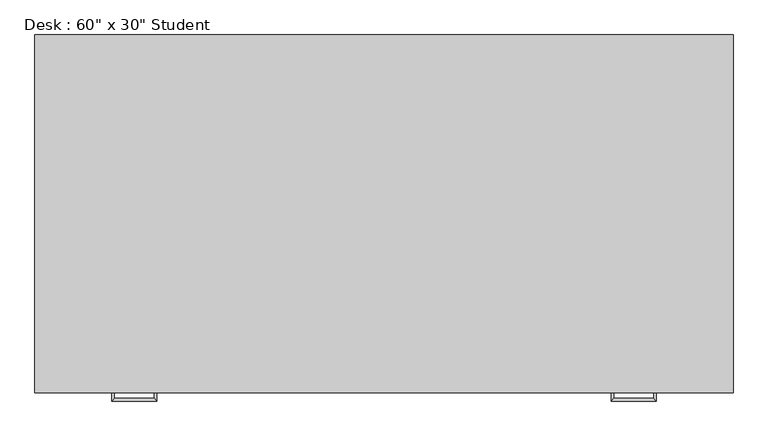
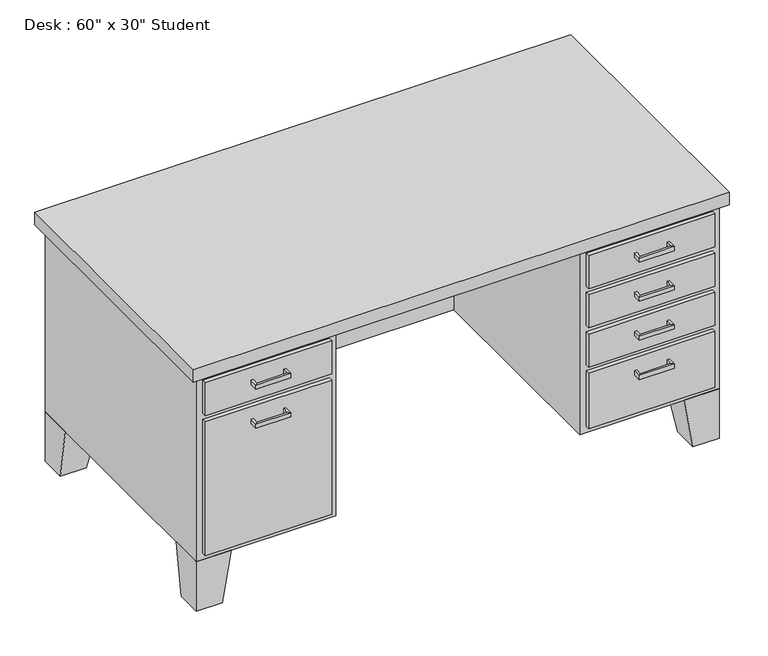
"""IFC4 building model written with IfcOpenShell, lengths in millimetres: furniture geometry."""

from ifc_helpers import new_model, si_unit, frame, origin, place, context, project, spatial, polyline, outline, extrude, faceted_brep, source, transform, mapped, element, save


def furniture_013ab306(model_context):
    return source(origin(), model_context, "Body", "SolidModel", [
        extrude(outline(polyline([(19.05, 0.0), (387.35, 0.0), (387.35, -12.7), (19.05, -12.7), (19.05, 0.0)])), frame((0.0, 0.0, 603.25), z_axis=(0.0, 0.0, 1.0), x_axis=(1.0, 0.0, 0.0)), (0.0, 0.0, 1.0), 101.6),
        extrude(outline(polyline([(19.05, 0.0), (387.35, 0.0), (387.35, -12.7), (19.05, -12.7), (19.05, 0.0)])), frame((0.0, 0.0, 171.45), z_axis=(0.0, 0.0, 1.0), x_axis=(1.0, 0.0, 0.0)), (0.0, 0.0, 1.0), 412.75),
        extrude(outline(polyline([(1136.65, 0.0), (1504.95, 0.0), (1504.95, -12.7), (1136.65, -12.7), (1136.65, 0.0)])), frame((0.0, 0.0, 603.25), z_axis=(0.0, 0.0, 1.0), x_axis=(1.0, 0.0, 0.0)), (0.0, 0.0, 1.0), 101.6),
        extrude(outline(polyline([(1136.65, 0.0), (1504.95, 0.0), (1504.95, -12.7), (1136.65, -12.7), (1136.65, 0.0)])), frame((0.0, 0.0, 171.45), z_axis=(0.0, 0.0, 1.0), x_axis=(1.0, 0.0, 0.0)), (0.0, 0.0, 1.0), 171.45),
        extrude(outline(polyline([(1136.65, 0.0), (1504.95, 0.0), (1504.95, -12.7), (1136.65, -12.7), (1136.65, 0.0)])), frame((0.0, 0.0, 482.6), z_axis=(0.0, 0.0, 1.0), x_axis=(1.0, 0.0, 0.0)), (0.0, 0.0, 1.0), 101.6),
        extrude(outline(polyline([(1136.65, 0.0), (1504.95, 0.0), (1504.95, -12.7), (1136.65, -12.7), (1136.65, 0.0)])), frame((0.0, 0.0, 361.95), z_axis=(0.0, 0.0, 1.0), x_axis=(1.0, 0.0, 0.0)), (0.0, 0.0, 1.0), 101.6),
        faceted_brep([(101.6, 0.0, 152.4), (101.6, 101.6, 152.4), (0.0, 101.6, 152.4), (0.0, 0.0, 152.4), (76.2, 0.0, 0.0), (0.0, 0.0, 0.0), (0.0, 76.2, 0.0), (76.2, 76.2, 0.0)], [[[0, 1, 2, 3]], [[4, 5, 6, 7]], [[4, 7, 1, 0]], [[7, 6, 2, 1]], [[6, 5, 3, 2]], [[5, 4, 0, 3]]]),
        faceted_brep([(101.6, 762.0, 152.4), (0.0, 762.0, 152.4), (0.0, 660.4, 152.4), (101.6, 660.4, 152.4), (76.2, 762.0, 0.0), (76.2, 685.8, 0.0), (0.0, 685.8, 0.0), (0.0, 762.0, 0.0)], [[[0, 1, 2, 3]], [[4, 5, 6, 7]], [[4, 7, 1, 0]], [[7, 6, 2, 1]], [[6, 5, 3, 2]], [[5, 4, 0, 3]]]),
        faceted_brep([(1422.4, 762.0, 152.4), (1422.4, 660.4, 152.4), (1524.0, 660.4, 152.4), (1524.0, 762.0, 152.4), (1447.8, 762.0, 0.0), (1524.0, 762.0, 0.0), (1524.0, 685.8, 0.0), (1447.8, 685.8, 0.0)], [[[0, 1, 2, 3]], [[4, 5, 6, 7]], [[4, 7, 1, 0]], [[7, 6, 2, 1]], [[6, 5, 3, 2]], [[5, 4, 0, 3]]]),
        faceted_brep([(1422.4, 0.0, 152.4), (1524.0, 0.0, 152.4), (1524.0, 101.6, 152.4), (1422.4, 101.6, 152.4), (1447.8, 0.0, 0.0), (1447.8, 76.2, 0.0), (1524.0, 76.2, 0.0), (1524.0, 0.0, 0.0)], [[[0, 1, 2, 3]], [[4, 5, 6, 7]], [[4, 7, 1, 0]], [[7, 6, 2, 1]], [[6, 5, 3, 2]], [[5, 4, 0, 3]]]),
        extrude(outline(polyline([(-19.05, -19.05), (-19.05, 781.05), (1543.05, 781.05), (1543.05, -19.05), (-19.05, -19.05)])), frame((0.0, 0.0, 723.9), z_axis=(0.0, 0.0, 1.0), x_axis=(1.0, 0.0, 0.0)), (0.0, 0.0, 1.0), 38.1),
        extrude(outline(polyline([(1117.6, 0.0), (1117.6, 635.0), (406.4, 635.0), (406.4, 0.0), (0.0, 0.0), (0.0, 762.0), (1524.0, 762.0), (1524.0, 0.0), (1117.6, 0.0)])), frame((0.0, 0.0, 152.4), z_axis=(0.0, 0.0, 1.0), x_axis=(1.0, 0.0, 0.0)), (0.0, 0.0, 1.0), 571.5),
        faceted_brep([(158.75, -12.7, 546.1), (158.75, -12.7, 533.4), (152.4, -12.7, 533.4), (152.4, -12.7, 546.1), (158.75, -31.75, 546.1), (158.75, -31.75, 533.4), (152.4, -38.1, 533.4), (152.4, -38.1, 546.1), (247.65, -31.75, 546.1), (247.65, -31.75, 533.4), (254.0, -38.1, 533.4), (254.0, -38.1, 546.1), (247.65, -12.7, 546.1), (254.0, -12.7, 546.1), (254.0, -12.7, 533.4), (247.65, -12.7, 533.4)], [[[0, 1, 2, 3]], [[1, 0, 4, 5]], [[2, 1, 5, 6]], [[3, 2, 6, 7]], [[0, 3, 7, 4]], [[5, 4, 8, 9]], [[6, 5, 9, 10]], [[7, 6, 10, 11]], [[4, 7, 11, 8]], [[12, 13, 14, 15]], [[9, 8, 12, 15]], [[10, 9, 15, 14]], [[11, 10, 14, 13]], [[8, 11, 13, 12]]]),
        faceted_brep([(158.75, -12.7, 666.75), (158.75, -12.7, 654.05), (152.4, -12.7, 654.05), (152.4, -12.7, 666.75), (158.75, -31.75, 666.75), (158.75, -31.75, 654.05), (152.4, -38.1, 654.05), (152.4, -38.1, 666.75), (247.65, -31.75, 666.75), (247.65, -31.75, 654.05), (254.0, -38.1, 654.05), (254.0, -38.1, 666.75), (247.65, -12.7, 666.75), (254.0, -12.7, 666.75), (254.0, -12.7, 654.05), (247.65, -12.7, 654.05)], [[[0, 1, 2, 3]], [[1, 0, 4, 5]], [[2, 1, 5, 6]], [[3, 2, 6, 7]], [[0, 3, 7, 4]], [[5, 4, 8, 9]], [[6, 5, 9, 10]], [[7, 6, 10, 11]], [[4, 7, 11, 8]], [[12, 13, 14, 15]], [[9, 8, 12, 15]], [[10, 9, 15, 14]], [[11, 10, 14, 13]], [[8, 11, 13, 12]]]),
        faceted_brep([(1365.25, -12.7, 304.8), (1371.6, -12.7, 304.8), (1371.6, -12.7, 292.1), (1365.25, -12.7, 292.1), (1365.25, -31.75, 304.8), (1371.6, -38.1, 304.8), (1371.6, -38.1, 292.1), (1365.25, -31.75, 292.1), (1276.35, -31.75, 304.8), (1270.0, -38.1, 304.8), (1270.0, -38.1, 292.1), (1276.35, -31.75, 292.1), (1276.35, -12.7, 304.8), (1276.35, -12.7, 292.1), (1270.0, -12.7, 292.1), (1270.0, -12.7, 304.8)], [[[0, 1, 2, 3]], [[1, 0, 4, 5]], [[2, 1, 5, 6]], [[3, 2, 6, 7]], [[0, 3, 7, 4]], [[5, 4, 8, 9]], [[6, 5, 9, 10]], [[7, 6, 10, 11]], [[4, 7, 11, 8]], [[12, 13, 14, 15]], [[9, 8, 12, 15]], [[10, 9, 15, 14]], [[11, 10, 14, 13]], [[8, 11, 13, 12]]]),
        faceted_brep([(1365.25, -12.7, 425.45), (1371.6, -12.7, 425.45), (1371.6, -12.7, 412.75), (1365.25, -12.7, 412.75), (1365.25, -31.75, 425.45), (1371.6, -38.1, 425.45), (1371.6, -38.1, 412.75), (1365.25, -31.75, 412.75), (1276.35, -31.75, 425.45), (1270.0, -38.1, 425.45), (1270.0, -38.1, 412.75), (1276.35, -31.75, 412.75), (1276.35, -12.7, 425.45), (1276.35, -12.7, 412.75), (1270.0, -12.7, 412.75), (1270.0, -12.7, 425.45)], [[[0, 1, 2, 3]], [[1, 0, 4, 5]], [[2, 1, 5, 6]], [[3, 2, 6, 7]], [[0, 3, 7, 4]], [[5, 4, 8, 9]], [[6, 5, 9, 10]], [[7, 6, 10, 11]], [[4, 7, 11, 8]], [[12, 13, 14, 15]], [[9, 8, 12, 15]], [[10, 9, 15, 14]], [[11, 10, 14, 13]], [[8, 11, 13, 12]]]),
        faceted_brep([(1365.25, -12.7, 546.1), (1371.6, -12.7, 546.1), (1371.6, -12.7, 533.4), (1365.25, -12.7, 533.4), (1365.25, -31.75, 546.1), (1371.6, -38.1, 546.1), (1371.6, -38.1, 533.4), (1365.25, -31.75, 533.4), (1276.35, -31.75, 546.1), (1270.0, -38.1, 546.1), (1270.0, -38.1, 533.4), (1276.35, -31.75, 533.4), (1276.35, -12.7, 546.1), (1276.35, -12.7, 533.4), (1270.0, -12.7, 533.4), (1270.0, -12.7, 546.1)], [[[0, 1, 2, 3]], [[1, 0, 4, 5]], [[2, 1, 5, 6]], [[3, 2, 6, 7]], [[0, 3, 7, 4]], [[5, 4, 8, 9]], [[6, 5, 9, 10]], [[7, 6, 10, 11]], [[4, 7, 11, 8]], [[12, 13, 14, 15]], [[9, 8, 12, 15]], [[10, 9, 15, 14]], [[11, 10, 14, 13]], [[8, 11, 13, 12]]]),
        faceted_brep([(1365.25, -12.7, 666.75), (1371.6, -12.7, 666.75), (1371.6, -12.7, 654.05), (1365.25, -12.7, 654.05), (1365.25, -31.75, 666.75), (1371.6, -38.1, 666.75), (1371.6, -38.1, 654.05), (1365.25, -31.75, 654.05), (1276.35, -31.75, 666.75), (1270.0, -38.1, 666.75), (1270.0, -38.1, 654.05), (1276.35, -31.75, 654.05), (1276.35, -12.7, 666.75), (1276.35, -12.7, 654.05), (1270.0, -12.7, 654.05), (1270.0, -12.7, 666.75)], [[[0, 1, 2, 3]], [[1, 0, 4, 5]], [[2, 1, 5, 6]], [[3, 2, 6, 7]], [[0, 3, 7, 4]], [[5, 4, 8, 9]], [[6, 5, 9, 10]], [[7, 6, 10, 11]], [[4, 7, 11, 8]], [[12, 13, 14, 15]], [[9, 8, 12, 15]], [[10, 9, 15, 14]], [[11, 10, 14, 13]], [[8, 11, 13, 12]]]),
    ])


if __name__ == "__main__":
    model = new_model("IFC4")
    model_context = context("Model", 3, world=origin())
    ifc_project = project(units=[si_unit("LENGTHUNIT", "METRE", prefix="MILLI")], contexts=[model_context])
    site = spatial("IfcSite", under=ifc_project)
    building = spatial("IfcBuilding", under=site)
    placement = place(None, origin())
    furniture_shape = furniture_013ab306(model_context)
    element("IfcFurniture", 1, ObjectType="Desk : 60\" x 30\" Student", at=placement, inside=building, context=model_context, shape_type="MappedRepresentation", body=[
        mapped(furniture_shape, transform((0.0, 0.0, 0.0), x_axis=(1.0, 0.0, 0.0), y_axis=(0.0, 1.0, 0.0), z_axis=(0.0, 0.0, 1.0))),
    ])
    save(model, "model.ifc")

# Revit data of these elements
# Type "Desk : 60\" x 30\" Student"
#   Assembly Code = "E2020200"
#   Depth = 2' - 6"
#   Height = 2' - 6"
#   Leg Height = 0' - 6"
#   Width = 5' - 0"
#   Body Material = Laminate, Ivory, Matte
#   Handle/Leg Material = Steel, Chrome Plated
#   Top Material = Cherry
#   Default Elevation = 0
# Element 1 (IfcFurniture, "Desk : 60\" x 30\" Student")
#   Materials on its faces: "Steel, Chrome Plated", "Laminate, Ivory, Matte", "Cherry"
# Materials
#   "Laminate, Ivory, Matte": class "Plastic", colour RGB 247 247 239, transparency 0, Description = "Plastic Laminate - Ivory, Matte", Cost = 0
#   "Steel, Chrome Plated": class "Metal", colour RGB 17 17 17, transparency 0, Description = "Chromiuim plated steel", Cost = 0
#   "Cherry": class "Wood", colour RGB 226 177 128, transparency 0, Description = "Prunus Serotina", Cost = 0
